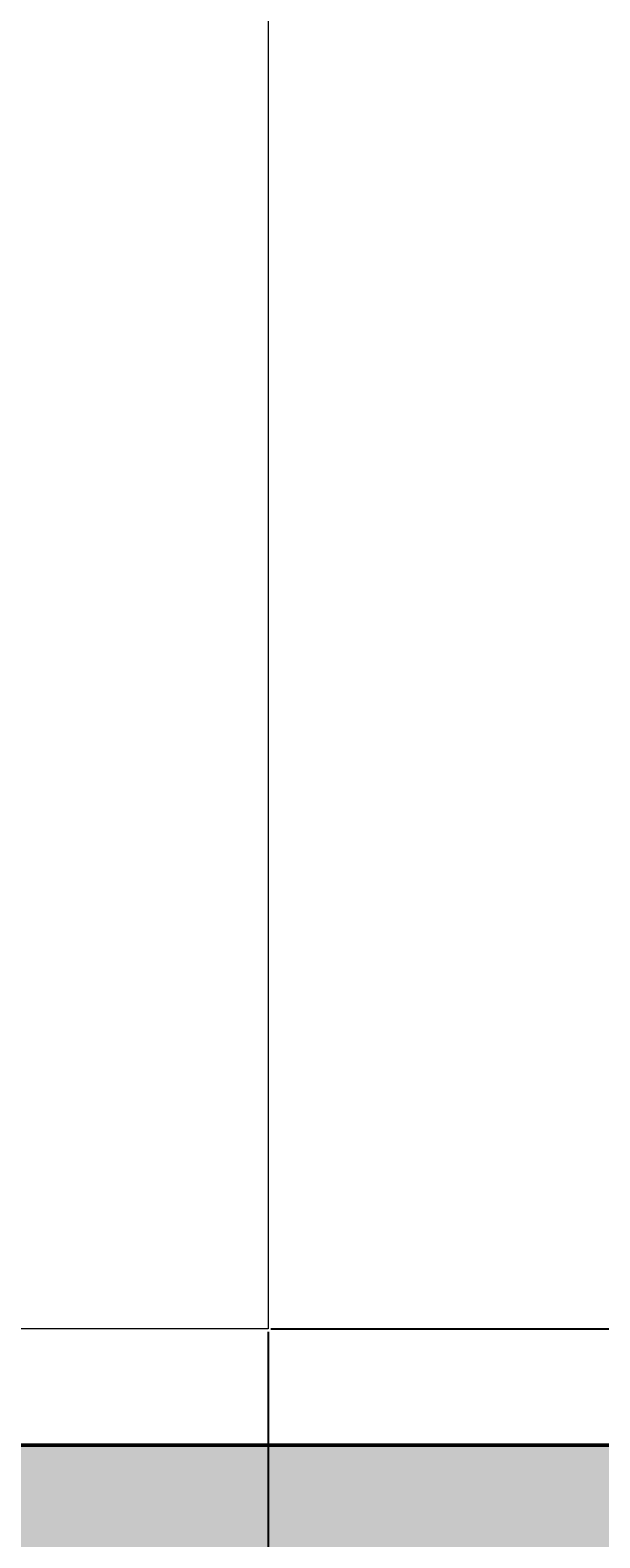
# Model space of a CAD drawing. Units: inches. Extents: x 2231 to 2461, y 2045 to 2455.
# Tile 45 of 95: x 2336 to 2348, y 2185 to 2217. Entities that reach past the tile are written whole.
import ezdxf

# ---------------------------------------------------------------- set-up
doc = ezdxf.new("R2010")
doc.units = ezdxf.units.IN
for name, color, linetype, lineweight in [('A-ANNO-DIMS', 2, 'Continuous', 18), ('A-FURN', 9, 'Continuous', 18), ('A-WALL', 7, 'Continuous', 50)]:
    doc.layers.add(name, color=color, linetype=linetype, lineweight=lineweight)
doc.layers.add('A-WALL-PATT', color=18, linetype='Continuous', lineweight=13, true_color=0x000000)
doc.styles.get("Standard").update_dxf_attribs({"font": 'arial.ttf'})
doc.dimstyles.get("Standard").update_dxf_attribs({"dimtxt": 0.18, "dimasz": 0.18, "dimexe": 0.18, "dimexo": 0.0625, "dimgap": 0.09, "dimtad": 0, "dimtih": 1, "dimtoh": 1, "dimdec": 4, "dimzin": 0, "dimdsep": 46, "dimtxsty": 'Standard', "dimcen": 0.09, "dimadec": 0, "dimazin": 0, "dimtfac": 1, "dimtdec": 4, "dimtofl": 0, "dimtmove": 0, "dimatfit": 3, "dimfxl": 1, "dimtolj": 1, "dimtzin": 0, "dimarcsym": 0})

# ---------------------------------------------------------------- blocks, each defined once
blk = doc.blocks.new('*D52')
at = {"layer": 'A-ANNO-DIMS', "color": 0, "lineweight": -2, "transparency": 16777216}
for p, q in [((2330.794, 2306.77), (2330.794, 2044.803)), ((2360.794, 2306.77), (2360.794, 2044.803)), ((2330.974, 2044.983), (2345.575, 2044.983)), ((2360.614, 2044.983), (2346.012, 2044.983))]:
    blk.add_line(p, q, dxfattribs=at)
at = {"layer": 'A-ANNO-DIMS', "color": 0, "transparency": 16777216}
for points in [[(2330.974, 2045.013), (2330.974, 2044.953), (2330.794, 2044.983)], [(2360.614, 2045.013), (2360.614, 2044.953), (2360.794, 2044.983)]]:
    blk.add_solid(points, dxfattribs=at)
at = {"layer": 'Defpoints', "color": 0, "transparency": 16777216}
for p in [(2330.794, 2306.833), (2360.794, 2306.833), (2360.794, 2044.983)]:
    blk.add_point(p, dxfattribs=at)
at = {"layer": 'A-ANNO-DIMS', "color": 0, "transparency": 16777216, "insert": (2345.794, 2044.983), "char_height": 0.18, "attachment_point": 5}
blk.add_mtext('\\A1;30', dxfattribs=at)
blk = doc.blocks.new('*D64')
at = {"layer": 'A-ANNO-DIMS', "color": 0, "lineweight": -2, "transparency": 16777216}
for p, q in [((2340.73, 2261.358), (2359.48, 2261.358)), ((2359.3, 2261.178), (2359.3, 2225.535)), ((2359.3, 2189.528), (2359.3, 2225.171)), ((2340.73, 2189.348), (2359.48, 2189.348))]:
    blk.add_line(p, q, dxfattribs=at)
at = {"layer": 'A-ANNO-DIMS', "color": 0, "transparency": 16777216}
for points in [[(2359.27, 2261.178), (2359.33, 2261.178), (2359.3, 2261.358)], [(2359.27, 2189.528), (2359.33, 2189.528), (2359.3, 2189.348)]]:
    blk.add_solid(points, dxfattribs=at)
at = {"layer": 'Defpoints', "color": 0, "transparency": 16777216}
for p in [(2340.667, 2261.358), (2340.667, 2189.348), (2359.3, 2189.348)]:
    blk.add_point(p, dxfattribs=at)
at = {"layer": 'A-ANNO-DIMS', "color": 0, "transparency": 16777216, "insert": (2359.3, 2225.353), "char_height": 0.18, "attachment_point": 5}
blk.add_mtext('\\A1;72.01', dxfattribs=at)
blk = doc.blocks.new('*D65')
at = {"layer": 'A-ANNO-DIMS', "color": 0, "lineweight": -2, "transparency": 16777216}
for p, q in [((2285.635, 2189.285), (2285.635, 2044.803)), ((2340.667, 2189.285), (2340.667, 2044.803)), ((2285.815, 2044.983), (2312.758, 2044.983)), ((2340.487, 2044.983), (2313.545, 2044.983))]:
    blk.add_line(p, q, dxfattribs=at)
at = {"layer": 'A-ANNO-DIMS', "color": 0, "transparency": 16777216}
for points in [[(2285.815, 2045.013), (2285.815, 2044.953), (2285.635, 2044.983)], [(2340.487, 2045.013), (2340.487, 2044.953), (2340.667, 2044.983)]]:
    blk.add_solid(points, dxfattribs=at)
at = {"layer": 'Defpoints', "color": 0, "transparency": 16777216}
for p in [(2285.635, 2189.348), (2340.667, 2189.348), (2340.667, 2044.983)]:
    blk.add_point(p, dxfattribs=at)
at = {"layer": 'A-ANNO-DIMS', "color": 0, "transparency": 16777216, "insert": (2313.151, 2044.983), "char_height": 0.18, "attachment_point": 5}
blk.add_mtext('\\A1;55.03', dxfattribs=at)
blk = doc.blocks.new('*D69')
at = {"layer": 'A-ANNO-DIMS', "color": 0, "lineweight": -2, "transparency": 16777216}
for p, q in [((2340.667, 2189.285), (2340.667, 2044.803)), ((2394.794, 2186.77), (2394.794, 2044.803)), ((2340.847, 2044.983), (2367.337, 2044.983)), ((2394.614, 2044.983), (2368.124, 2044.983))]:
    blk.add_line(p, q, dxfattribs=at)
at = {"layer": 'A-ANNO-DIMS', "color": 0, "transparency": 16777216}
for points in [[(2340.847, 2045.013), (2340.847, 2044.953), (2340.667, 2044.983)], [(2394.614, 2045.013), (2394.614, 2044.953), (2394.794, 2044.983)]]:
    blk.add_solid(points, dxfattribs=at)
at = {"layer": 'Defpoints', "color": 0, "transparency": 16777216}
for p in [(2340.667, 2189.348), (2394.794, 2186.833), (2394.794, 2044.983)]:
    blk.add_point(p, dxfattribs=at)
at = {"layer": 'A-ANNO-DIMS', "color": 0, "transparency": 16777216, "insert": (2367.73, 2044.983), "char_height": 0.18, "attachment_point": 5}
blk.add_mtext('\\A1;54.13', dxfattribs=at)

msp = doc.modelspace()

# ---------------------------------------------------------------- hatches: boundary and pattern name
at = {"layer": 'A-WALL-PATT'}
h = msp.add_hatch(color=256, dxfattribs=at)
h.dxf.hatch_style = 1
h.paths.add_polyline_path([(2441.7935, 2269.1535), (2432.7935, 2269.1535), (2432.7935, 2186.8328), (2396.7935, 2186.8328), (2396.7935, 2286.8328), (2394.7935, 2286.8328), (2394.7935, 2186.8328), (2334.7935, 2186.8328), (2334.7935, 2182.8328), (2432.7935, 2182.8328), (2432.7935, 2072.8328), (2416.6639, 2072.8328), (2416.6639, 2063.8328), (2441.7935, 2063.8328)])
h.paths.add_polyline_path([(2368.6639, 2072.8328), (2367.04, 2072.8328), (2330.7942, 2072.8328), (2330.7397, 2063.8328), (2368.6639, 2063.8328)])
h.paths.add_polyline_path([(2300.7392, 2068.3328), (2300.7392, 2072.8328), (2298.7935, 2072.8328), (2294.7935, 2072.8328), (2258.7935, 2072.8328), (2258.7935, 2120.8328), (2294.7935, 2120.8328), (2298.7935, 2120.8328), (2298.7935, 2128.8328), (2294.7935, 2128.8328), (2294.7935, 2124.8328), (2258.7935, 2124.8328), (2258.7935, 2182.8328), (2294.7935, 2182.8328), (2294.7935, 2174.8328), (2298.7935, 2174.8328), (2298.7935, 2182.8328), (2304.7935, 2182.8328), (2304.7935, 2186.8328), (2258.7935, 2186.8328), (2258.7935, 2221.999), (2249.7935, 2221.999), (2249.7935, 2063.8328), (2300.7392, 2063.8328)])
h.paths.add_polyline_path([(2391.9338, 2435.8328), (2333.82, 2435.8328), (2333.82, 2426.8328), (2368.7935, 2426.8328), (2368.7935, 2374.9508), (2368.7935, 2370.8328), (2372.3935, 2370.8328), (2372.7935, 2370.8328), (2372.7935, 2426.8328), (2391.9338, 2426.8328)])
h.paths.add_polyline_path([(2441.7935, 2435.8328), (2415.9338, 2435.8328), (2415.9338, 2426.8328), (2432.7935, 2426.8328), (2432.7935, 2334.8328), (2372.7935, 2334.8328), (2372.7935, 2346.8328), (2368.7935, 2346.8328), (2368.7935, 2306.8328), (2360.7935, 2306.8328), (2360.7935, 2302.8328), (2368.7935, 2302.8328), (2372.7935, 2302.8328), (2372.7935, 2330.8328), (2432.7935, 2330.8328), (2432.7935, 2317.1535), (2441.7935, 2317.1535)])
h.paths.add_polyline_path([(2285.82, 2435.8328), (2249.7935, 2435.8328), (2249.7935, 2269.999), (2258.7935, 2269.999), (2258.7935, 2302.8328), (2318.8168, 2302.8328), (2330.7935, 2302.8328), (2330.7935, 2306.8328), (2258.7935, 2306.8328), (2258.7935, 2426.8328), (2285.82, 2426.8328)])

# ---------------------------------------------------------------- linework, layer by layer
at = {"layer": 'A-FURN'}
msp.add_lwpolyline([(2285.6353, 2255.1137), (2285.6353, 2261.3584), (2340.6673, 2261.3584), (2340.6673, 2189.3477), (2285.6353, 2189.3477), (2285.6353, 2195.1137)], dxfattribs=at)
at = {"layer": 'A-WALL'}
msp.add_line((2334.7935, 2186.8328), (2394.7935, 2186.8328), dxfattribs=at)

# ---------------------------------------------------------------- dimensions: what is measured, and where the dimension line sits
at = {"layer": 'A-ANNO-DIMS'}
for base, p1, p2, override, picture, middle in [((2360.7935, 2044.9825), (2330.7935, 2306.8328), (2360.7935, 2306.8328), {"dimdec": 0, "dimlfac": 1, "dimrnd": 0, "dimzin": 0, "dimdsep": 46, "dimlunit": 2}, '*D52', (2345.7935, 2044.9825)), ((2340.6673, 2044.9825), (2285.6353, 2189.3477), (2340.6673, 2189.3477), {"dimdec": 2, "dimlfac": 1, "dimrnd": 0, "dimzin": 0, "dimdsep": 46, "dimlunit": 2}, '*D65', (2313.1513, 2044.9825)), ((2394.7935, 2044.9825), (2340.6673, 2189.3477), (2394.7935, 2186.8328), {"dimdec": 2, "dimlfac": 1, "dimrnd": 0, "dimzin": 0, "dimdsep": 46, "dimlunit": 2}, '*D69', (2367.7304, 2044.9825))]:
    dim = msp.add_linear_dim(base=base, p1=p1, p2=p2, dimstyle='Standard', override=override, dxfattribs=at)
    dim.commit()
    dim.dimension.update_dxf_attribs({"geometry": picture, "text_midpoint": middle})
dim = msp.add_linear_dim(base=(2359.2998, 2189.3477), p1=(2340.6673, 2261.3584), p2=(2340.6673, 2189.3477), angle=270, dimstyle='Standard', override={"dimdec": 2, "dimlfac": 1, "dimrnd": 0, "dimzin": 0, "dimdsep": 46, "dimlunit": 2}, dxfattribs=at)
dim.commit()
dim.dimension.update_dxf_attribs({"geometry": '*D64', "text_midpoint": (2359.2998, 2225.353)})

doc.saveas('drawing.dxf')
